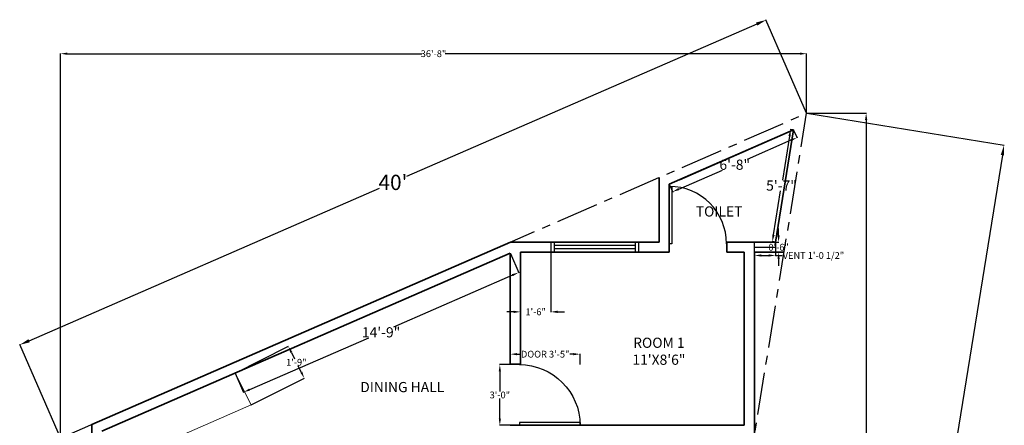
# Model space of a CAD drawing. Units: inches. Extents: x 1778 to 2384, y 384 to 1080.
# Tile 3 of 3: x 1804 to 2384, y 841 to 1080. Entities that reach past the tile are written whole.
import ezdxf

# ---------------------------------------------------------------- set-up
doc = ezdxf.new("R2010")
doc.units = ezdxf.units.IN
doc.header["$MEASUREMENT"] = 0
doc.linetypes.add('CENTER', pattern=[2, 1.25, -0.25, 0.25, -0.25])
for name, color, linetype, lineweight in [('A-ANNO-DIMS', 2, 'Continuous', 18), ('A-AREA-IDEN', 1, 'Continuous', 18), ('A-FLOR-FIXT', 8, 'Continuous', 18), ('A-GLAZ', 4, 'Continuous', 18), ('A-WALL', 7, 'Continuous', 35), ('C-PROP', 13, 'CENTER', 25), ('DOOR', 13, 'Continuous', 25)]:
    doc.layers.add(name, color=color, linetype=linetype, lineweight=lineweight)
doc.styles.get("Standard").update_dxf_attribs({"font": 'arial.ttf'})
doc.dimstyles.get("Standard").update_dxf_attribs({"dimtxt": 4, "dimasz": 4, "dimexe": 0.18, "dimexo": 0.0625, "dimgap": 0.09, "dimtad": 0, "dimtih": 1, "dimtoh": 1, "dimdec": 0, "dimzin": 0, "dimdsep": 46, "dimlunit": 3, "dimtxsty": 'Standard', "dimcen": 0.09, "dimadec": 0, "dimazin": 0, "dimtfac": 1, "dimtdec": 0, "dimtofl": 0, "dimtmove": 0, "dimatfit": 3, "dimfxl": 1, "dimtolj": 1, "dimtzin": 0, "dimarcsym": 0})

# ---------------------------------------------------------------- blocks, each defined once
blk = doc.blocks.new('*D1')
at = {"layer": 'A-ANNO-DIMS', "color": 0, "lineweight": -2, "transparency": 16777216}
for p, q in [((2267.72, 1024.58), (2384.25, 1005.72)), ((2383.11, 999.82), (2341.67, 743.88)), ((2298.72, 478.61), (2340.16, 734.55)), ((2181.42, 491.52), (2297.94, 472.66))]:
    blk.add_line(p, q, dxfattribs=at)
at = {"layer": 'A-ANNO-DIMS', "color": 0, "transparency": 16777216}
for points in [[(2382.12, 999.98), (2384.1, 999.66), (2384.07, 1005.75)], [(2297.74, 478.77), (2299.71, 478.45), (2297.77, 472.69)]]:
    blk.add_solid(points, dxfattribs=at)
at = {"layer": 'Defpoints', "color": 0, "transparency": 16777216}
for p in [(2267.66, 1024.59), (2384.07, 1005.75), (2181.36, 491.53)]:
    blk.add_point(p, dxfattribs=at)
at = {"layer": 'A-ANNO-DIMS', "color": 0, "transparency": 16777216, "insert": (2340.92, 739.22), "char_height": 9, "attachment_point": 5}
blk.add_mtext("\\A1;45'", dxfattribs=at)
blk = doc.blocks.new('*D4')
at = {"layer": 'A-ANNO-DIMS', "color": 0, "lineweight": -2, "transparency": 16777216}
for p, q in [((2238.23, 1077.18), (2031.58, 987.25)), ((2267.63, 1024.65), (2243.66, 1079.74)), ((1809.1, 890.44), (2015.76, 980.36)), ((1827.5, 833.12), (1803.53, 888.21))]:
    blk.add_line(p, q, dxfattribs=at)
at = {"layer": 'A-ANNO-DIMS', "color": 0, "transparency": 16777216}
for points in [[(2237.83, 1078.09), (2238.63, 1076.26), (2243.73, 1079.57)], [(1808.7, 891.35), (1809.5, 889.52), (1803.6, 888.04)]]:
    blk.add_solid(points, dxfattribs=at)
at = {"layer": 'Defpoints', "color": 0, "transparency": 16777216}
for p in [(2243.73, 1079.57), (2267.66, 1024.59), (1827.53, 833.06)]:
    blk.add_point(p, dxfattribs=at)
at = {"layer": 'A-ANNO-DIMS', "color": 0, "transparency": 16777216, "insert": (2023.67, 983.81), "char_height": 9, "attachment_point": 5}
blk.add_mtext("\\A1;40'", dxfattribs=at)
blk = doc.blocks.new('*D5')
at = {"layer": 'A-ANNO-DIMS', "color": 0, "lineweight": -2, "transparency": 16777216}
for p, q in [((2260.01, 1014.65), (2262.01, 1010.04)), ((2258.27, 1008.61), (2232.51, 997.39)), ((2192.25, 979.88), (2218.02, 991.09)), ((2186.65, 982.73), (2188.66, 978.12))]:
    blk.add_line(p, q, dxfattribs=at)
at = {"layer": 'A-ANNO-DIMS', "color": 0, "transparency": 16777216}
for points in [[(2258.01, 1009.22), (2258.54, 1007.99), (2261.94, 1010.2)], [(2191.99, 980.49), (2192.52, 979.27), (2188.59, 978.28)]]:
    blk.add_solid(points, dxfattribs=at)
at = {"layer": 'Defpoints', "color": 0, "transparency": 16777216}
for p in [(2259.98, 1014.71), (2261.94, 1010.2), (2186.63, 982.79)]:
    blk.add_point(p, dxfattribs=at)
at = {"layer": 'A-ANNO-DIMS', "color": 0, "transparency": 16777216, "insert": (2225.26, 994.24), "char_height": 6, "attachment_point": 5}
blk.add_mtext('\\A1;6\'-8"', dxfattribs=at)
blk = doc.blocks.new('*D7')
at = {"layer": 'A-ANNO-DIMS', "color": 0, "lineweight": -2, "transparency": 16777216}
for p, q in [((2092.92, 941.94), (2097.89, 930.52)), ((2094.15, 929.09), (2023.91, 898.53)), ((1939.18, 861.66), (2009.42, 892.22)), ((1930.62, 871.31), (1935.59, 859.9))]:
    blk.add_line(p, q, dxfattribs=at)
at = {"layer": 'A-ANNO-DIMS', "color": 0, "transparency": 16777216}
for points in [[(2093.88, 929.7), (2094.41, 928.48), (2097.81, 930.69)], [(1938.92, 862.27), (1939.45, 861.05), (1935.52, 860.06)]]:
    blk.add_solid(points, dxfattribs=at)
at = {"layer": 'Defpoints', "color": 0, "transparency": 16777216}
for p in [(2092.89, 942), (2097.81, 930.69), (1930.6, 871.37)]:
    blk.add_point(p, dxfattribs=at)
at = {"layer": 'A-ANNO-DIMS', "color": 0, "transparency": 16777216, "insert": (2016.67, 895.38), "char_height": 6, "attachment_point": 5}
blk.add_mtext('\\A1;14\'-9"', dxfattribs=at)
blk = doc.blocks.new('*D10')
at = {"layer": 'A-ANNO-DIMS', "color": 0, "lineweight": -2, "transparency": 16777216}
for p, q in [((2257.55, 1011.05), (2253.34, 985.07)), ((2259.92, 1014.72), (2258.01, 1015.03)), ((2248.12, 952.81), (2252.33, 978.79)), ((2249.21, 948.58), (2247.3, 948.89))]:
    blk.add_line(p, q, dxfattribs=at)
at = {"layer": 'A-ANNO-DIMS', "color": 0, "transparency": 16777216}
for points in [[(2256.89, 1011.16), (2258.21, 1010.94), (2258.19, 1015)], [(2247.46, 952.91), (2248.78, 952.7), (2247.48, 948.86)]]:
    blk.add_solid(points, dxfattribs=at)
at = {"layer": 'Defpoints', "color": 0, "transparency": 16777216}
for p in [(2259.98, 1014.71), (2247.48, 948.86), (2249.27, 948.57)]:
    blk.add_point(p, dxfattribs=at)
at = {"layer": 'A-ANNO-DIMS', "color": 0, "transparency": 16777216, "insert": (2252.83, 981.93), "char_height": 6, "attachment_point": 5}
blk.add_mtext('\\A1;5\'-7"', dxfattribs=at)
blk = doc.blocks.new('*U14')
for p, q in [((0, 0), (0, -6)), ((40, 0), (40, -6))]:
    blk.add_line(p, q)
blk.add_lwpolyline([(0, 0), (0, 40), (1.75, 40), (1.75, 0)], close=True)
blk.add_arc((0, 0), 40, 0, 90)
blk = doc.blocks.new('DOOR')
blk.add_blockref('*U14', (1810.9, 983.44))
blk = doc.blocks.new('WINDOW')
for p, q in [((1664.47, 998.33), (1658.47, 998.33)), ((1658.47, 950.33), (1664.47, 950.33))]:
    blk.add_line(p, q)
at = {"layer": 'DOOR'}
for p, q in [((1664.47, 1000.33), (1658.47, 1000.33)), ((1660.47, 998.33), (1660.47, 950.33)), ((1662.47, 998.33), (1662.47, 950.33)), ((1658.47, 948.33), (1664.47, 948.33))]:
    blk.add_line(p, q, dxfattribs=at)
blk = doc.blocks.new('WIN')
at = {"layer": 'Defpoints'}
for p, q in [((1658.47, 1000.33), (1658.47, 948.33)), ((1664.47, 1000.33), (1664.47, 948.33))]:
    blk.add_line(p, q, dxfattribs=at)
at = {"layer": 'DOOR'}
blk.add_blockref('WINDOW', (0, 0), dxfattribs=at)
blk = doc.blocks.new('V3')
at = {"layer": 'Defpoints'}
for p, q in [((2236.89, 948.57), (2249.27, 948.57)), ((2249.27, 942.57), (2236.89, 942.57))]:
    blk.add_line(p, q, dxfattribs=at)
at = {"layer": 'DOOR'}
for p, q in [((2236.89, 942.57), (2236.89, 948.57)), ((2249.27, 948.57), (2249.27, 942.57)), ((2236.89, 945.57), (2249.27, 945.57))]:
    blk.add_line(p, q, dxfattribs=at)
blk = doc.blocks.new('*D25')
at = {"layer": 'A-ANNO-DIMS', "color": 0, "lineweight": -2, "transparency": 16777216}
for p, q in [((2092.89, 876.4), (2092.89, 882.69)), ((2134.03, 876.4), (2134.03, 882.69)), ((2096.89, 882.51), (2099, 882.51)), ((2130.03, 882.51), (2127.93, 882.51))]:
    blk.add_line(p, q, dxfattribs=at)
at = {"layer": 'A-ANNO-DIMS', "color": 0, "transparency": 16777216}
for points in [[(2096.89, 883.18), (2096.89, 881.85), (2092.89, 882.51)], [(2130.03, 883.18), (2130.03, 881.85), (2134.03, 882.51)]]:
    blk.add_solid(points, dxfattribs=at)
at = {"layer": 'Defpoints', "color": 0, "transparency": 16777216}
for p in [(2134.03, 882.51), (2092.89, 876.34), (2134.03, 876.34)]:
    blk.add_point(p, dxfattribs=at)
at = {"layer": 'A-ANNO-DIMS', "color": 0, "transparency": 16777216, "insert": (2113.46, 882.51), "char_height": 4, "attachment_point": 5}
blk.add_mtext('\\A1;DOOR 3\'-5"', dxfattribs=at)
blk = doc.blocks.new('*D26')
at = {"layer": 'A-ANNO-DIMS', "color": 0, "lineweight": -2, "transparency": 16777216}
for p, q in [((2092.83, 876.34), (2086.54, 876.34)), ((2086.72, 872.34), (2086.72, 860.59)), ((2086.72, 844.57), (2086.72, 856.32)), ((2092.83, 840.57), (2086.54, 840.57))]:
    blk.add_line(p, q, dxfattribs=at)
at = {"layer": 'A-ANNO-DIMS', "color": 0, "transparency": 16777216}
for points in [[(2086.06, 872.34), (2087.39, 872.34), (2086.72, 876.34)], [(2086.06, 844.57), (2087.39, 844.57), (2086.72, 840.57)]]:
    blk.add_solid(points, dxfattribs=at)
at = {"layer": 'Defpoints', "color": 0, "transparency": 16777216}
for p in [(2086.72, 876.34), (2092.89, 876.34), (2092.89, 840.57)]:
    blk.add_point(p, dxfattribs=at)
at = {"layer": 'A-ANNO-DIMS', "color": 0, "transparency": 16777216, "insert": (2086.72, 858.46), "char_height": 4, "attachment_point": 5}
blk.add_mtext('\\A1;3\'-0"', dxfattribs=at)
blk = doc.blocks.new('*D33')
at = {"layer": 'A-ANNO-DIMS', "color": 0, "lineweight": -2, "transparency": 16777216}
for p, q in [((2236.89, 942.51), (2236.89, 940.53)), ((2249.27, 942.51), (2249.27, 940.53)), ((2240.89, 940.71), (2245.27, 940.71)), ((2249.27, 940.71), (2253.27, 940.71))]:
    blk.add_line(p, q, dxfattribs=at)
at = {"layer": 'A-ANNO-DIMS', "color": 0, "transparency": 16777216}
for points in [[(2240.89, 941.38), (2240.89, 940.05), (2236.89, 940.71)], [(2245.27, 941.38), (2245.27, 940.05), (2249.27, 940.71)]]:
    blk.add_solid(points, dxfattribs=at)
at = {"layer": 'Defpoints', "color": 0, "transparency": 16777216}
for p in [(2236.89, 942.57), (2249.27, 942.57), (2249.27, 940.71)]:
    blk.add_point(p, dxfattribs=at)
at = {"layer": 'A-ANNO-DIMS', "color": 0, "transparency": 16777216, "insert": (2271.67, 940.71), "char_height": 4, "attachment_point": 5}
blk.add_mtext('\\A1;VENT 1\'-0 1/2"', dxfattribs=at)
blk = doc.blocks.new('*D34')
at = {"layer": 'A-ANNO-DIMS', "color": 0, "lineweight": -2, "transparency": 16777216}
for p, q in [((2251.13, 952.57), (2251.13, 956.57)), ((2249.33, 948.57), (2251.31, 948.57)), ((2249.33, 942.57), (2251.31, 942.57)), ((2251.13, 938.57), (2251.13, 934.57))]:
    blk.add_line(p, q, dxfattribs=at)
at = {"layer": 'A-ANNO-DIMS', "color": 0, "transparency": 16777216}
for points in [[(2250.46, 952.57), (2251.8, 952.57), (2251.13, 948.57)], [(2250.46, 938.57), (2251.8, 938.57), (2251.13, 942.57)]]:
    blk.add_solid(points, dxfattribs=at)
at = {"layer": 'Defpoints', "color": 0, "transparency": 16777216}
for p in [(2249.27, 948.57), (2251.13, 948.57), (2249.27, 942.57)]:
    blk.add_point(p, dxfattribs=at)
at = {"layer": 'A-ANNO-DIMS', "color": 0, "transparency": 16777216, "insert": (2251.13, 945.57), "char_height": 4, "attachment_point": 5}
blk.add_mtext('\\A1;0\'-6"', dxfattribs=at)
blk = doc.blocks.new('*D35')
at = {"layer": 'A-ANNO-DIMS', "color": 0, "lineweight": -2, "transparency": 16777216}
for p, q in [((2267.72, 1024.59), (2302.94, 1024.59)), ((2302.76, 1020.59), (2302.76, 760.19)), ((2302.76, 495.53), (2302.76, 755.94)), ((2181.42, 491.53), (2302.94, 491.53))]:
    blk.add_line(p, q, dxfattribs=at)
at = {"layer": 'A-ANNO-DIMS', "color": 0, "transparency": 16777216}
for points in [[(2302.09, 1020.59), (2303.43, 1020.59), (2302.76, 1024.59)], [(2302.09, 495.53), (2303.43, 495.53), (2302.76, 491.53)]]:
    blk.add_solid(points, dxfattribs=at)
at = {"layer": 'Defpoints', "color": 0, "transparency": 16777216}
for p in [(2267.66, 1024.59), (2302.76, 1024.59), (2181.36, 491.53)]:
    blk.add_point(p, dxfattribs=at)
at = {"layer": 'A-ANNO-DIMS', "color": 0, "transparency": 16777216, "insert": (2302.76, 758.06), "char_height": 4, "attachment_point": 5}
blk.add_mtext('\\A1;44\'-5"', dxfattribs=at)
blk = doc.blocks.new('*D36')
at = {"layer": 'A-ANNO-DIMS', "color": 0, "lineweight": -2, "transparency": 16777216}
for p, q in [((1827.53, 833.13), (1827.53, 1059.87)), ((1831.53, 1059.69), (2040.63, 1059.69)), ((2263.66, 1059.69), (2054.55, 1059.69)), ((2267.66, 1024.66), (2267.66, 1059.87))]:
    blk.add_line(p, q, dxfattribs=at)
at = {"layer": 'A-ANNO-DIMS', "color": 0, "transparency": 16777216}
for points in [[(1831.53, 1060.36), (1831.53, 1059.03), (1827.53, 1059.69)], [(2263.66, 1060.36), (2263.66, 1059.03), (2267.66, 1059.69)]]:
    blk.add_solid(points, dxfattribs=at)
at = {"layer": 'Defpoints', "color": 0, "transparency": 16777216}
for p in [(2267.66, 1059.69), (2267.66, 1024.59), (1827.53, 833.06)]:
    blk.add_point(p, dxfattribs=at)
at = {"layer": 'A-ANNO-DIMS', "color": 0, "transparency": 16777216, "insert": (2047.59, 1059.69), "char_height": 4, "attachment_point": 5}
blk.add_mtext('\\A1;36\'-8"', dxfattribs=at)
blk = doc.blocks.new('*D41')
at = {"layer": 'A-ANNO-DIMS', "color": 0, "lineweight": -2, "transparency": 16777216}
for p, q in [((2098.89, 942.51), (2098.89, 907.29)), ((2116.76, 942.51), (2116.76, 907.29)), ((2094.89, 907.47), (2090.89, 907.47)), ((2120.76, 907.47), (2124.76, 907.47))]:
    blk.add_line(p, q, dxfattribs=at)
at = {"layer": 'A-ANNO-DIMS', "color": 0, "transparency": 16777216}
for points in [[(2094.89, 908.14), (2094.89, 906.8), (2098.89, 907.47)], [(2120.76, 908.14), (2120.76, 906.8), (2116.76, 907.47)]]:
    blk.add_solid(points, dxfattribs=at)
at = {"layer": 'Defpoints', "color": 0, "transparency": 16777216}
for p in [(2098.89, 942.57), (2116.76, 942.57), (2098.89, 907.47)]:
    blk.add_point(p, dxfattribs=at)
at = {"layer": 'A-ANNO-DIMS', "color": 0, "transparency": 16777216, "insert": (2107.83, 907.47), "char_height": 4, "attachment_point": 5}
blk.add_mtext('\\A1;1\'-6"', dxfattribs=at)
blk = doc.blocks.new('*D46')
at = {"layer": 'A-ANNO-DIMS', "color": 0, "lineweight": -2, "transparency": 16777216}
for p, q in [((1930.65, 871.4), (1962.12, 887.2)), ((1963.76, 883.55), (1965.61, 879.86)), ((1969.61, 871.9), (1967.75, 875.59)), ((1940.09, 852.6), (1971.56, 868.41))]:
    blk.add_line(p, q, dxfattribs=at)
at = {"layer": 'A-ANNO-DIMS', "color": 0, "transparency": 16777216}
for points in [[(1964.35, 883.85), (1963.16, 883.25), (1961.96, 887.12)], [(1970.2, 872.2), (1969.01, 871.6), (1971.4, 868.33)]]:
    blk.add_solid(points, dxfattribs=at)
at = {"layer": 'Defpoints', "color": 0, "transparency": 16777216}
for p in [(1930.6, 871.37), (1971.4, 868.33), (1940.03, 852.58)]:
    blk.add_point(p, dxfattribs=at)
at = {"layer": 'A-ANNO-DIMS', "color": 0, "transparency": 16777216, "insert": (1966.68, 877.73), "char_height": 4, "attachment_point": 5}
blk.add_mtext('\\A1;1\'-9"', dxfattribs=at)

msp = doc.modelspace()

# ---------------------------------------------------------------- linework, layer by layer
at = {"layer": 'A-FLOR-FIXT'}
msp.add_line((1930.6, 871.37), (1940.03, 852.58), dxfattribs=at)
at = {"layer": 'A-FLOR-FIXT', "ltscale": 20}
msp.add_line((1873.03, 823.42), (1940.03, 852.58), dxfattribs=at)
at = {"layer": 'A-WALL'}
for p, q in [((2259.98, 1014.71), (2186.63, 982.79)), ((2259.98, 1014.71), (2249.27, 948.57)), ((2259.98, 1014.71), (2249.27, 948.57)), ((2180.63, 986.72), (2180.63, 948.57)), ((2186.63, 982.79), (2186.63, 942.57)), ((1846.03, 841.12), (2092.96, 948.57)), ((2180.63, 948.57), (2092.96, 948.57)), ((2249.27, 948.57), (2220.63, 948.57)), ((2220.63, 948.57), (2220.63, 942.57)), ((2092.89, 876.57), (2092.89, 942)), ((2098.89, 876.57), (2098.89, 942.57)), ((2186.63, 942.57), (2098.89, 942.57)), ((2230.89, 942.57), (2220.63, 942.57)), ((2230.89, 840.57), (2230.89, 942.57)), ((2254.38, 942.57), (2236.89, 942.57)), ((2236.89, 834.57), (2236.89, 942.57)), ((2098.89, 876.57), (2092.89, 876.57)), ((1846.03, 777.54), (1846.03, 841.12)), ((2098.89, 840.57), (2092.89, 840.57)), ((2230.89, 840.57), (2098.89, 840.57))]:
    msp.add_line(p, q, dxfattribs=at)
at = {"layer": 'A-WALL', "ltscale": 20}
for p, q in [((2192.63, 985.4), (2259.98, 1014.71)), ((1852.03, 837.18), (2092.89, 942))]:
    msp.add_line(p, q, dxfattribs=at)
at = {"layer": 'C-PROP', "ltscale": 20}
for p in [(1827.53, 833.06), (2181.36, 491.53)]:
    msp.add_line(p, (2267.66, 1024.59), dxfattribs=at)

# ---------------------------------------------------------------- block references
at = {"layer": 'A-GLAZ', "rotation": 270}
msp.add_blockref('WIN', (1168.43, 2607.04), dxfattribs=at)
at = {"layer": 'A-GLAZ'}
msp.add_blockref('V3', (0, 0), dxfattribs=at)
at = {"layer": 'DOOR', "xscale": 0.8447881913510608, "yscale": 0.8447881913510608, "zscale": 0.8447881913510608}
msp.add_blockref('DOOR', (656.79, 116.84), dxfattribs=at)
at = {"layer": 'DOOR', "xscale": -0.8943109005136252, "yscale": 0.8943109005136252, "zscale": 0.8943109005136252, "rotation": 270}
msp.add_blockref('DOOR', (1218.76, -778.94), dxfattribs=at)

# ---------------------------------------------------------------- texts
at = {"layer": 'A-AREA-IDEN', "char_height": 6}
for s, insert, attachment_point in [('TOILET', (2202.27, 969.65), 1), ('ROOM 1\\P11\'X8\'6"', (2180.53, 892.24), 2), ('DINING HALL', (2004.37, 866.11), 1)]:
    msp.add_mtext_dynamic_manual_height_columns(s, width=72.6444, gutter_width=1, heights=[0], dxfattribs=dict(at, insert=insert, attachment_point=attachment_point))

# ---------------------------------------------------------------- dimensions: what is measured, and where the dimension line sits
at = {"layer": 'A-ANNO-DIMS'}
for p1, p2, distance, override, picture, middle in [((1827.53, 833.06), (2267.66, 1024.59), 59.96, {"dimtxt": 9, "dimasz": 6, "dimclrd": 0, "dimclre": 0, "dimclrt": 0}, '*D4', (2023.67, 983.81)), ((2181.36, 491.53), (2267.66, 1024.59), -117.92, {"dimtxt": 9, "dimasz": 6, "dimclrd": 0, "dimclre": 0, "dimclrt": 0}, '*D1', (2340.92, 739.22)), ((2186.63, 982.79), (2259.98, 1014.71), -4.91, {"dimtxt": 6, "dimclrd": 0, "dimclre": 0, "dimclrt": 0}, '*D5', (2225.26, 994.24)), ((2259.98, 1014.71), (2249.27, 948.57), -1.81, {"dimtxt": 6, "dimclrd": 0, "dimclre": 0, "dimclrt": 0}, '*D10', (2252.83, 981.93)), ((1930.6, 871.37), (2092.89, 942), -12.33, {"dimtxt": 6, "dimclrd": 0, "dimclre": 0, "dimclrt": 0}, '*D7', (2016.67, 895.38))]:
    dim = msp.add_aligned_dim(p1=p1, p2=p2, distance=distance, dimstyle='Standard', override=override, dxfattribs=at)
    dim.commit()
    dim.dimension.update_dxf_attribs({"geometry": picture, "text_midpoint": middle})
dim = msp.add_linear_dim(base=(2267.66, 1059.69), p1=(1827.53, 833.06), p2=(2267.66, 1024.59), dimstyle='Standard', override={"dimdec": 1, "dimlfac": 1, "dimrnd": 0, "dimzin": 1, "dimdsep": 46, "dimlunit": 4, "dimfrac": 2}, dxfattribs=at)
dim.commit()
dim.dimension.update_dxf_attribs({"geometry": '*D36', "text_midpoint": (2047.59, 1059.69)})
for base, p1, p2, angle, picture, middle in [((2302.76, 1024.59), (2181.36, 491.53), (2267.66, 1024.59), 90, '*D35', (2302.76, 758.06)), ((2251.13, 948.57), (2249.27, 942.57), (2249.27, 948.57), 90, '*D34', (2251.13, 945.57)), ((2098.89, 907.47), (2116.76, 942.57), (2098.89, 942.57), 180, '*D41', (2107.83, 907.47)), ((1971.4, 868.33), (1930.6, 871.37), (1940.03, 852.58), 296.66457, '*D46', (1966.68, 877.73)), ((2086.72, 876.34), (2092.89, 840.57), (2092.89, 876.34), 90, '*D26', (2086.72, 858.46))]:
    dim = msp.add_linear_dim(base=base, p1=p1, p2=p2, angle=angle, dimstyle='Standard', override={"dimdec": 1, "dimlfac": 1, "dimrnd": 0, "dimzin": 1, "dimdsep": 46, "dimlunit": 4, "dimfrac": 2}, dxfattribs=at)
    dim.commit()
    dim.dimension.update_dxf_attribs({"geometry": picture, "text_midpoint": middle})
for base, p1, p2, text, picture, middle in [((2249.27, 940.71), (2236.89, 942.57), (2249.27, 942.57), 'VENT <>', '*D33', (2271.67, 940.71)), ((2134.03, 882.51), (2092.89, 876.34), (2134.03, 876.34), 'DOOR <>', '*D25', (2113.46, 882.51))]:
    dim = msp.add_linear_dim(base=base, p1=p1, p2=p2, text=text, dimstyle='Standard', override={"dimdec": 1, "dimlfac": 1, "dimrnd": 0, "dimzin": 1, "dimdsep": 46, "dimlunit": 4, "dimfrac": 2}, dxfattribs=at)
    dim.commit()
    dim.dimension.update_dxf_attribs({"geometry": picture, "text_midpoint": middle})

doc.saveas('drawing.dxf')
